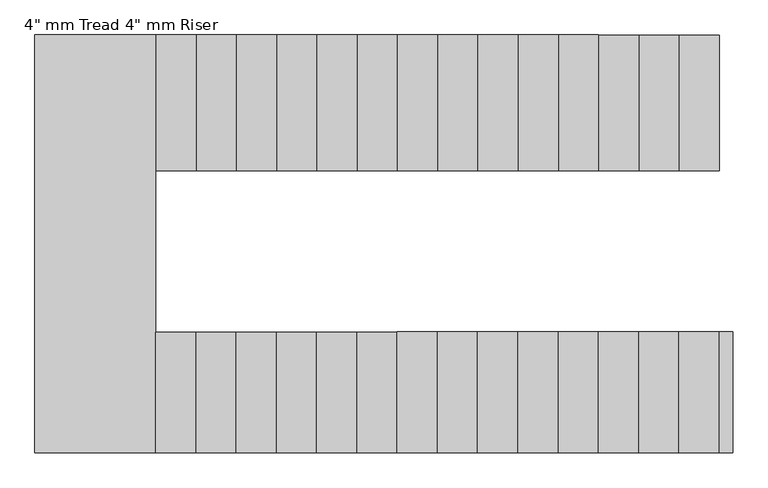
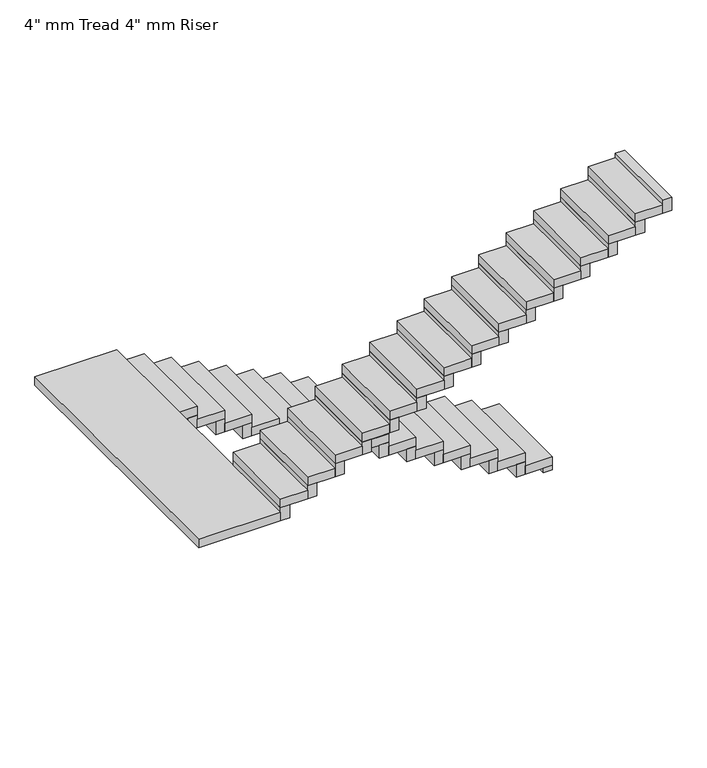
"""IFC4 building model written with IfcOpenShell, lengths in millimetres: stair flight geometry."""

from ifc_helpers import new_model, si_unit, frame, origin, origin_with_axes, place, context, project, spatial, polyline, outline, extrude, source, transform, mapped, element, save


def stair_flight_2352bd75(model_context):
    return source(origin(), model_context, "Body", "SweptSolid", [
        extrude(outline(polyline([(-12061.2412437, -28173.9205555), (-11959.6412437, -28173.9205555), (-11959.6412437, -29202.6205555), (-12061.2412437, -29202.6205555), (-12061.2412437, -28173.9205555)])), origin_with_axes(), (0.0, 0.0, 1.0), 50.8),
        extrude(outline(polyline([(-12264.4412437, -29202.6205555), (-12264.4412437, -28173.9205555), (-11959.6412437, -28173.9205555), (-11959.6412437, -29202.6205555), (-12264.4412437, -29202.6205555)])), frame((0.0, 0.0, 50.8), z_axis=(0.0, 0.0, 1.0), x_axis=(1.0, 0.0, 0.0)), (0.0, 0.0, 1.0), 101.6),
        extrude(outline(polyline([(-12366.0412437, -28173.9205555), (-12264.4412437, -28173.9205555), (-12264.4412437, -29202.6205555), (-12366.0412437, -29202.6205555), (-12366.0412437, -28173.9205555)])), frame((0.0, 0.0, 50.8), z_axis=(0.0, 0.0, 1.0), x_axis=(1.0, 0.0, 0.0)), (0.0, 0.0, 1.0), 152.4),
        extrude(outline(polyline([(-12569.2412437, -29202.6205555), (-12569.2412437, -28173.9205555), (-12264.4412437, -28173.9205555), (-12264.4412437, -29202.6205555), (-12569.2412437, -29202.6205555)])), frame((0.0, 0.0, 203.2), z_axis=(0.0, 0.0, 1.0), x_axis=(1.0, 0.0, 0.0)), (0.0, 0.0, 1.0), 101.6),
        extrude(outline(polyline([(-12670.8412437, -28173.9205555), (-12569.2412437, -28173.9205555), (-12569.2412437, -29202.6205555), (-12670.8412437, -29202.6205555), (-12670.8412437, -28173.9205555)])), frame((0.0, 0.0, 203.2), z_axis=(0.0, 0.0, 1.0), x_axis=(1.0, 0.0, 0.0)), (0.0, 0.0, 1.0), 152.4),
        extrude(outline(polyline([(-12874.0412437, -29202.6205555), (-12874.0412437, -28173.9205555), (-12569.2412437, -28173.9205555), (-12569.2412437, -29202.6205555), (-12874.0412437, -29202.6205555)])), frame((0.0, 0.0, 355.6), z_axis=(0.0, 0.0, 1.0), x_axis=(1.0, 0.0, 0.0)), (0.0, 0.0, 1.0), 101.6),
        extrude(outline(polyline([(-12975.6412437, -28173.9205555), (-12874.0412437, -28173.9205555), (-12874.0412437, -29202.6205555), (-12975.6412437, -29202.6205555), (-12975.6412437, -28173.9205555)])), frame((0.0, 0.0, 355.6), z_axis=(0.0, 0.0, 1.0), x_axis=(1.0, 0.0, 0.0)), (0.0, 0.0, 1.0), 152.4),
        extrude(outline(polyline([(-13178.8412437, -29202.6205555), (-13178.8412437, -28173.9205555), (-12874.0412437, -28173.9205555), (-12874.0412437, -29202.6205555), (-13178.8412437, -29202.6205555)])), frame((0.0, 0.0, 508.0), z_axis=(0.0, 0.0, 1.0), x_axis=(1.0, 0.0, 0.0)), (0.0, 0.0, 1.0), 101.6),
        extrude(outline(polyline([(-13280.4412437, -28173.9205555), (-13178.8412437, -28173.9205555), (-13178.8412437, -29202.6205555), (-13280.4412437, -29202.6205555), (-13280.4412437, -28173.9205555)])), frame((0.0, 0.0, 508.0), z_axis=(0.0, 0.0, 1.0), x_axis=(1.0, 0.0, 0.0)), (0.0, 0.0, 1.0), 152.4),
        extrude(outline(polyline([(-13483.6412437, -29202.6205555), (-13483.6412437, -28173.9205555), (-13178.8412437, -28173.9205555), (-13178.8412437, -29202.6205555), (-13483.6412437, -29202.6205555)])), frame((0.0, 0.0, 660.4), z_axis=(0.0, 0.0, 1.0), x_axis=(1.0, 0.0, 0.0)), (0.0, 0.0, 1.0), 101.6),
        extrude(outline(polyline([(-13585.2412437, -28173.9205555), (-13483.6412437, -28173.9205555), (-13483.6412437, -29202.6205555), (-13585.2412437, -29202.6205555), (-13585.2412437, -28173.9205555)])), frame((0.0, 0.0, 660.4), z_axis=(0.0, 0.0, 1.0), x_axis=(1.0, 0.0, 0.0)), (0.0, 0.0, 1.0), 152.4),
        extrude(outline(polyline([(-13788.4412437, -29202.6205555), (-13788.4412437, -28173.9205555), (-13483.6412437, -28173.9205555), (-13483.6412437, -29202.6205555), (-13788.4412437, -29202.6205555)])), frame((0.0, 0.0, 812.8), z_axis=(0.0, 0.0, 1.0), x_axis=(1.0, 0.0, 0.0)), (0.0, 0.0, 1.0), 101.6),
        extrude(outline(polyline([(-13890.0412437, -28173.9205555), (-13788.4412437, -28173.9205555), (-13788.4412437, -29202.6205555), (-13890.0412437, -29202.6205555), (-13890.0412437, -28173.9205555)])), frame((0.0, 0.0, 812.8), z_axis=(0.0, 0.0, 1.0), x_axis=(1.0, 0.0, 0.0)), (0.0, 0.0, 1.0), 152.4),
        extrude(outline(polyline([(-14093.2412437, -29202.6205555), (-14093.2412437, -28173.9205555), (-13788.4412437, -28173.9205555), (-13788.4412437, -29202.6205555), (-14093.2412437, -29202.6205555)])), frame((0.0, 0.0, 965.2), z_axis=(0.0, 0.0, 1.0), x_axis=(1.0, 0.0, 0.0)), (0.0, 0.0, 1.0), 101.6),
        extrude(outline(polyline([(-14194.8412437, -28173.9205555), (-14093.2412437, -28173.9205555), (-14093.2412437, -29202.6205555), (-14194.8412437, -29202.6205555), (-14194.8412437, -28173.9205555)])), frame((0.0, 0.0, 965.2), z_axis=(0.0, 0.0, 1.0), x_axis=(1.0, 0.0, 0.0)), (0.0, 0.0, 1.0), 152.4),
        extrude(outline(polyline([(-14398.0412437, -29202.6205555), (-14398.0412437, -28173.9205555), (-14093.2412437, -28173.9205555), (-14093.2412437, -29202.6205555), (-14398.0412437, -29202.6205555)])), frame((0.0, 0.0, 1117.6), z_axis=(0.0, 0.0, 1.0), x_axis=(1.0, 0.0, 0.0)), (0.0, 0.0, 1.0), 101.6),
        extrude(outline(polyline([(-14499.6412437, -28173.9205555), (-14398.0412437, -28173.9205555), (-14398.0412437, -29202.6205555), (-14499.6412437, -29202.6205555), (-14499.6412437, -28173.9205555)])), frame((0.0, 0.0, 1117.6), z_axis=(0.0, 0.0, 1.0), x_axis=(1.0, 0.0, 0.0)), (0.0, 0.0, 1.0), 152.4),
        extrude(outline(polyline([(-14702.8412437, -29202.6205555), (-14702.8412437, -28173.9205555), (-14398.0412437, -28173.9205555), (-14398.0412437, -29202.6205555), (-14702.8412437, -29202.6205555)])), frame((0.0, 0.0, 1270.0), z_axis=(0.0, 0.0, 1.0), x_axis=(1.0, 0.0, 0.0)), (0.0, 0.0, 1.0), 101.6),
        extrude(outline(polyline([(-14804.4412437, -28173.9205555), (-14702.8412437, -28173.9205555), (-14702.8412437, -29202.6205555), (-14804.4412437, -29202.6205555), (-14804.4412437, -28173.9205555)])), frame((0.0, 0.0, 1270.0), z_axis=(0.0, 0.0, 1.0), x_axis=(1.0, 0.0, 0.0)), (0.0, 0.0, 1.0), 152.4),
        extrude(outline(polyline([(-15007.6412437, -29202.6205555), (-15007.6412437, -28173.9205555), (-14702.8412437, -28173.9205555), (-14702.8412437, -29202.6205555), (-15007.6412437, -29202.6205555)])), frame((0.0, 0.0, 1422.4), z_axis=(0.0, 0.0, 1.0), x_axis=(1.0, 0.0, 0.0)), (0.0, 0.0, 1.0), 101.6),
        extrude(outline(polyline([(-15109.2412437, -28173.9205555), (-15007.6412437, -28173.9205555), (-15007.6412437, -29202.6205555), (-15109.2412437, -29202.6205555), (-15109.2412437, -28173.9205555)])), frame((0.0, 0.0, 1422.4), z_axis=(0.0, 0.0, 1.0), x_axis=(1.0, 0.0, 0.0)), (0.0, 0.0, 1.0), 152.4),
        extrude(outline(polyline([(-15312.4412437, -29202.6205555), (-15312.4412437, -28173.9205555), (-15007.6412437, -28173.9205555), (-15007.6412437, -29202.6205555), (-15312.4412437, -29202.6205555)])), frame((0.0, 0.0, 1574.8), z_axis=(0.0, 0.0, 1.0), x_axis=(1.0, 0.0, 0.0)), (0.0, 0.0, 1.0), 101.6),
        extrude(outline(polyline([(-15414.0412437, -28173.9205555), (-15312.4412437, -28173.9205555), (-15312.4412437, -29202.6205555), (-15414.0412437, -29202.6205555), (-15414.0412437, -28173.9205555)])), frame((0.0, 0.0, 1574.8), z_axis=(0.0, 0.0, 1.0), x_axis=(1.0, 0.0, 0.0)), (0.0, 0.0, 1.0), 152.4),
        extrude(outline(polyline([(-15617.2412437, -29202.6205555), (-15617.2412437, -28173.9205555), (-15312.4412437, -28173.9205555), (-15312.4412437, -29202.6205555), (-15617.2412437, -29202.6205555)])), frame((0.0, 0.0, 1727.2), z_axis=(0.0, 0.0, 1.0), x_axis=(1.0, 0.0, 0.0)), (0.0, 0.0, 1.0), 101.6),
        extrude(outline(polyline([(-15718.8412437, -28173.9205555), (-15617.2412437, -28173.9205555), (-15617.2412437, -29202.6205555), (-15718.8412437, -29202.6205555), (-15718.8412437, -28173.9205555)])), frame((0.0, 0.0, 1727.2), z_axis=(0.0, 0.0, 1.0), x_axis=(1.0, 0.0, 0.0)), (0.0, 0.0, 1.0), 152.4),
        extrude(outline(polyline([(-15922.0412437, -29202.6205555), (-15922.0412437, -28173.9205555), (-15617.2412437, -28173.9205555), (-15617.2412437, -29202.6205555), (-15922.0412437, -29202.6205555)])), frame((0.0, 0.0, 1879.6), z_axis=(0.0, 0.0, 1.0), x_axis=(1.0, 0.0, 0.0)), (0.0, 0.0, 1.0), 101.6),
        extrude(outline(polyline([(-16023.6412437, -28173.9205555), (-15922.0412437, -28173.9205555), (-15922.0412437, -29202.6205555), (-16023.6412437, -29202.6205555), (-16023.6412437, -28173.9205555)])), frame((0.0, 0.0, 1879.6), z_axis=(0.0, 0.0, 1.0), x_axis=(1.0, 0.0, 0.0)), (0.0, 0.0, 1.0), 152.4),
        extrude(outline(polyline([(-16226.8412437, -29202.6205555), (-16226.8412437, -28173.9205555), (-15922.0412437, -28173.9205555), (-15922.0412437, -29202.6205555), (-16226.8412437, -29202.6205555)])), frame((0.0, 0.0, 2032.0), z_axis=(0.0, 0.0, 1.0), x_axis=(1.0, 0.0, 0.0)), (0.0, 0.0, 1.0), 101.6),
        extrude(outline(polyline([(-16328.4412437, -28173.9205555), (-16226.8412437, -28173.9205555), (-16226.8412437, -29202.6205555), (-16328.4412437, -29202.6205555), (-16328.4412437, -28173.9205555)])), frame((0.0, 0.0, 2032.0), z_axis=(0.0, 0.0, 1.0), x_axis=(1.0, 0.0, 0.0)), (0.0, 0.0, 1.0), 152.4),
        extrude(outline(polyline([(-16226.8412437, -30421.8205555), (-16226.8412437, -31336.2205555), (-17141.2412437, -31336.2205555), (-17141.2412437, -28173.9205555), (-16226.8412437, -28173.9205555), (-16226.8412437, -29202.6205555), (-16226.8412437, -30421.8205555)])), frame((0.0, 0.0, 2184.4), z_axis=(0.0, 0.0, 1.0), x_axis=(1.0, 0.0, 0.0)), (0.0, 0.0, 1.0), 101.6),
        extrude(outline(polyline([(-16125.2412437, -31336.2205555), (-16226.8412437, -31336.2205555), (-16226.8412437, -30421.8205555), (-16125.2412437, -30421.8205555), (-16125.2412437, -31336.2205555)])), frame((0.0, 0.0, 2184.4), z_axis=(0.0, 0.0, 1.0), x_axis=(1.0, 0.0, 0.0)), (0.0, 0.0, 1.0), 152.4),
        extrude(outline(polyline([(-15922.0412437, -30421.8205555), (-15922.0412437, -31336.2205555), (-16226.8412437, -31336.2205555), (-16226.8412437, -30421.8205555), (-15922.0412437, -30421.8205555)])), frame((0.0, 0.0, 2336.8), z_axis=(0.0, 0.0, 1.0), x_axis=(1.0, 0.0, 0.0)), (0.0, 0.0, 1.0), 101.6),
        extrude(outline(polyline([(-15820.4412437, -31336.2205555), (-15922.0412437, -31336.2205555), (-15922.0412437, -30421.8205555), (-15820.4412437, -30421.8205555), (-15820.4412437, -31336.2205555)])), frame((0.0, 0.0, 2336.8), z_axis=(0.0, 0.0, 1.0), x_axis=(1.0, 0.0, 0.0)), (0.0, 0.0, 1.0), 152.4),
        extrude(outline(polyline([(-15617.2412437, -30421.8205555), (-15617.2412437, -31336.2205555), (-15922.0412437, -31336.2205555), (-15922.0412437, -30421.8205555), (-15617.2412437, -30421.8205555)])), frame((0.0, 0.0, 2489.2), z_axis=(0.0, 0.0, 1.0), x_axis=(1.0, 0.0, 0.0)), (0.0, 0.0, 1.0), 101.6),
        extrude(outline(polyline([(-15515.6412437, -31336.2205555), (-15617.2412437, -31336.2205555), (-15617.2412437, -30421.8205555), (-15515.6412437, -30421.8205555), (-15515.6412437, -31336.2205555)])), frame((0.0, 0.0, 2489.2), z_axis=(0.0, 0.0, 1.0), x_axis=(1.0, 0.0, 0.0)), (0.0, 0.0, 1.0), 152.4),
        extrude(outline(polyline([(-15312.4412437, -30421.8205555), (-15312.4412437, -31336.2205555), (-15617.2412437, -31336.2205555), (-15617.2412437, -30421.8205555), (-15312.4412437, -30421.8205555)])), frame((0.0, 0.0, 2641.6), z_axis=(0.0, 0.0, 1.0), x_axis=(1.0, 0.0, 0.0)), (0.0, 0.0, 1.0), 101.6),
        extrude(outline(polyline([(-15210.8412437, -31336.2205555), (-15312.4412437, -31336.2205555), (-15312.4412437, -30421.8205555), (-15210.8412437, -30421.8205555), (-15210.8412437, -31336.2205555)])), frame((0.0, 0.0, 2641.6), z_axis=(0.0, 0.0, 1.0), x_axis=(1.0, 0.0, 0.0)), (0.0, 0.0, 1.0), 152.4),
        extrude(outline(polyline([(-15007.6412437, -30421.8205555), (-15007.6412437, -31336.2205555), (-15312.4412437, -31336.2205555), (-15312.4412437, -30421.8205555), (-15007.6412437, -30421.8205555)])), frame((0.0, 0.0, 2794.0), z_axis=(0.0, 0.0, 1.0), x_axis=(1.0, 0.0, 0.0)), (0.0, 0.0, 1.0), 101.6),
        extrude(outline(polyline([(-14906.0412437, -31336.2205555), (-15007.6412437, -31336.2205555), (-15007.6412437, -30421.8205555), (-14906.0412437, -30421.8205555), (-14906.0412437, -31336.2205555)])), frame((0.0, 0.0, 2794.0), z_axis=(0.0, 0.0, 1.0), x_axis=(1.0, 0.0, 0.0)), (0.0, 0.0, 1.0), 152.4),
        extrude(outline(polyline([(-14702.8412437, -30421.8205555), (-14702.8412437, -31336.2205555), (-15007.6412437, -31336.2205555), (-15007.6412437, -30421.8205555), (-14702.8412437, -30421.8205555)])), frame((0.0, 0.0, 2946.4), z_axis=(0.0, 0.0, 1.0), x_axis=(1.0, 0.0, 0.0)), (0.0, 0.0, 1.0), 101.6),
        extrude(outline(polyline([(-14601.2412437, -31336.2205555), (-14702.8412437, -31336.2205555), (-14702.8412437, -30421.8205555), (-14601.2412437, -30421.8205555), (-14601.2412437, -31336.2205555)])), frame((0.0, 0.0, 2946.4), z_axis=(0.0, 0.0, 1.0), x_axis=(1.0, 0.0, 0.0)), (0.0, 0.0, 1.0), 152.4),
        extrude(outline(polyline([(-14398.0412437, -30421.8205555), (-14398.0412437, -31336.2205555), (-14702.8412437, -31336.2205555), (-14702.8412437, -30421.8205555), (-14398.0412437, -30421.8205555)])), frame((0.0, 0.0, 3098.8), z_axis=(0.0, 0.0, 1.0), x_axis=(1.0, 0.0, 0.0)), (0.0, 0.0, 1.0), 101.6),
        extrude(outline(polyline([(-14296.4412437, -31336.2205555), (-14398.0412437, -31336.2205555), (-14398.0412437, -30421.8205555), (-14296.4412437, -30421.8205555), (-14296.4412437, -31336.2205555)])), frame((0.0, 0.0, 3098.8), z_axis=(0.0, 0.0, 1.0), x_axis=(1.0, 0.0, 0.0)), (0.0, 0.0, 1.0), 152.4),
        extrude(outline(polyline([(-14093.2412437, -30421.8205555), (-14093.2412437, -31336.2205555), (-14398.0412437, -31336.2205555), (-14398.0412437, -30421.8205555), (-14093.2412437, -30421.8205555)])), frame((0.0, 0.0, 3251.2), z_axis=(0.0, 0.0, 1.0), x_axis=(1.0, 0.0, 0.0)), (0.0, 0.0, 1.0), 101.6),
        extrude(outline(polyline([(-13991.6412437, -31336.2205555), (-14093.2412437, -31336.2205555), (-14093.2412437, -30421.8205555), (-13991.6412437, -30421.8205555), (-13991.6412437, -31336.2205555)])), frame((0.0, 0.0, 3251.2), z_axis=(0.0, 0.0, 1.0), x_axis=(1.0, 0.0, 0.0)), (0.0, 0.0, 1.0), 152.4),
        extrude(outline(polyline([(-13788.4412437, -30421.8205555), (-13788.4412437, -31336.2205555), (-14093.2412437, -31336.2205555), (-14093.2412437, -30421.8205555), (-13788.4412437, -30421.8205555)])), frame((0.0, 0.0, 3403.6), z_axis=(0.0, 0.0, 1.0), x_axis=(1.0, 0.0, 0.0)), (0.0, 0.0, 1.0), 101.6),
        extrude(outline(polyline([(-13686.8412437, -31336.2205555), (-13788.4412437, -31336.2205555), (-13788.4412437, -30421.8205555), (-13686.8412437, -30421.8205555), (-13686.8412437, -31336.2205555)])), frame((0.0, 0.0, 3403.6), z_axis=(0.0, 0.0, 1.0), x_axis=(1.0, 0.0, 0.0)), (0.0, 0.0, 1.0), 152.4),
        extrude(outline(polyline([(-13483.6412437, -30421.8205555), (-13483.6412437, -31336.2205555), (-13788.4412437, -31336.2205555), (-13788.4412437, -30421.8205555), (-13483.6412437, -30421.8205555)])), frame((0.0, 0.0, 3556.0), z_axis=(0.0, 0.0, 1.0), x_axis=(1.0, 0.0, 0.0)), (0.0, 0.0, 1.0), 101.6),
        extrude(outline(polyline([(-13382.0412437, -31336.2205555), (-13483.6412437, -31336.2205555), (-13483.6412437, -30421.8205555), (-13382.0412437, -30421.8205555), (-13382.0412437, -31336.2205555)])), frame((0.0, 0.0, 3556.0), z_axis=(0.0, 0.0, 1.0), x_axis=(1.0, 0.0, 0.0)), (0.0, 0.0, 1.0), 152.4),
        extrude(outline(polyline([(-13178.8412437, -30421.8205555), (-13178.8412437, -31336.2205555), (-13483.6412437, -31336.2205555), (-13483.6412437, -30421.8205555), (-13178.8412437, -30421.8205555)])), frame((0.0, 0.0, 3708.4), z_axis=(0.0, 0.0, 1.0), x_axis=(1.0, 0.0, 0.0)), (0.0, 0.0, 1.0), 101.6),
        extrude(outline(polyline([(-13077.2412437, -31336.2205555), (-13178.8412437, -31336.2205555), (-13178.8412437, -30421.8205555), (-13077.2412437, -30421.8205555), (-13077.2412437, -31336.2205555)])), frame((0.0, 0.0, 3708.4), z_axis=(0.0, 0.0, 1.0), x_axis=(1.0, 0.0, 0.0)), (0.0, 0.0, 1.0), 152.4),
        extrude(outline(polyline([(-12874.0412437, -30421.8205555), (-12874.0412437, -31336.2205555), (-13178.8412437, -31336.2205555), (-13178.8412437, -30421.8205555), (-12874.0412437, -30421.8205555)])), frame((0.0, 0.0, 3860.8), z_axis=(0.0, 0.0, 1.0), x_axis=(1.0, 0.0, 0.0)), (0.0, 0.0, 1.0), 101.6),
        extrude(outline(polyline([(-12772.4412437, -31336.2205555), (-12874.0412437, -31336.2205555), (-12874.0412437, -30421.8205555), (-12772.4412437, -30421.8205555), (-12772.4412437, -31336.2205555)])), frame((0.0, 0.0, 3860.8), z_axis=(0.0, 0.0, 1.0), x_axis=(1.0, 0.0, 0.0)), (0.0, 0.0, 1.0), 152.4),
        extrude(outline(polyline([(-12569.2412437, -30421.8205555), (-12569.2412437, -31336.2205555), (-12874.0412437, -31336.2205555), (-12874.0412437, -30421.8205555), (-12569.2412437, -30421.8205555)])), frame((0.0, 0.0, 4013.2), z_axis=(0.0, 0.0, 1.0), x_axis=(1.0, 0.0, 0.0)), (0.0, 0.0, 1.0), 101.6),
        extrude(outline(polyline([(-12467.6412437, -31336.2205555), (-12569.2412437, -31336.2205555), (-12569.2412437, -30421.8205555), (-12467.6412437, -30421.8205555), (-12467.6412437, -31336.2205555)])), frame((0.0, 0.0, 4013.2), z_axis=(0.0, 0.0, 1.0), x_axis=(1.0, 0.0, 0.0)), (0.0, 0.0, 1.0), 152.4),
        extrude(outline(polyline([(-12264.4412437, -30421.8205555), (-12264.4412437, -31336.2205555), (-12569.2412437, -31336.2205555), (-12569.2412437, -30421.8205555), (-12264.4412437, -30421.8205555)])), frame((0.0, 0.0, 4165.6), z_axis=(0.0, 0.0, 1.0), x_axis=(1.0, 0.0, 0.0)), (0.0, 0.0, 1.0), 101.6),
        extrude(outline(polyline([(-12162.8412437, -31336.2205555), (-12264.4412437, -31336.2205555), (-12264.4412437, -30421.8205555), (-12162.8412437, -30421.8205555), (-12162.8412437, -31336.2205555)])), frame((0.0, 0.0, 4165.6), z_axis=(0.0, 0.0, 1.0), x_axis=(1.0, 0.0, 0.0)), (0.0, 0.0, 1.0), 152.4),
        extrude(outline(polyline([(-11858.0412437, -31336.2205555), (-11959.6412437, -31336.2205555), (-11959.6412437, -30421.8205555), (-11858.0412437, -30421.8205555), (-11858.0412437, -31336.2205555)])), frame((0.0, 0.0, 4318.0), z_axis=(0.0, 0.0, 1.0), x_axis=(1.0, 0.0, 0.0)), (0.0, 0.0, 1.0), 152.4),
        extrude(outline(polyline([(-11959.6412437, -30421.8205555), (-11959.6412437, -31336.2205555), (-12264.4412437, -31336.2205555), (-12264.4412437, -30421.8205555), (-11959.6412437, -30421.8205555)])), frame((0.0, 0.0, 4318.0), z_axis=(0.0, 0.0, 1.0), x_axis=(1.0, 0.0, 0.0)), (0.0, 0.0, 1.0), 101.6),
    ])


if __name__ == "__main__":
    model = new_model("IFC4")
    model_context = context("Model", 3, world=origin())
    ifc_project = project(units=[si_unit("LENGTHUNIT", "METRE", prefix="MILLI")], contexts=[model_context])
    site = spatial("IfcSite", under=ifc_project)
    building = spatial("IfcBuilding", under=site)
    placement = place(None, origin())
    stair_flight_shape = stair_flight_2352bd75(model_context)
    element("IfcStairFlight", 1, ObjectType="4\" mm Tread 4\" mm Riser", at=placement, inside=building, context=model_context, shape_type="MappedRepresentation", body=[
        mapped(stair_flight_shape, transform((0.0, 0.0, 0.0), x_axis=(1.0, 0.0, 0.0), y_axis=(0.0, 1.0, 0.0), z_axis=(0.0, 0.0, 1.0))),
    ])
    save(model, "model.ifc")
